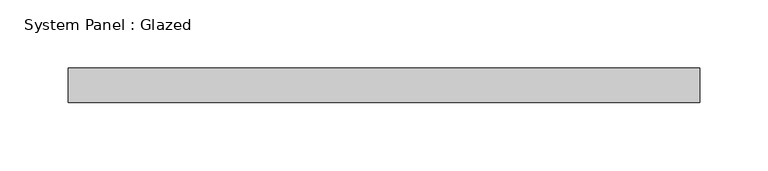
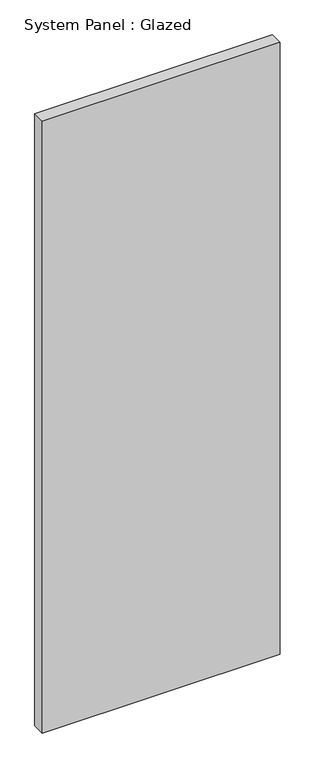
"""IFC4 building model written with IfcOpenShell, lengths in millimetres: plate geometry, System Panel : Glazed."""

from ifc_helpers import new_model, si_unit, origin, origin_with_axes, place, context, project, spatial, polyline, outline, extrude, source, transform, mapped, element, save


def system_panel_glazed_28e9ce38(model_context):
    return source(origin(), model_context, "Body", "SweptSolid", [
        extrude(outline(polyline([(231.775, 19.05), (-231.775, 19.05), (-231.775, 44.45), (231.775, 44.45), (231.775, 19.05)])), origin_with_axes(), (0.0, 0.0, 1.0), 1261.8321364),
    ])


if __name__ == "__main__":
    model = new_model("IFC4")
    model_context = context("Model", 3, world=origin())
    ifc_project = project(units=[si_unit("LENGTHUNIT", "METRE", prefix="MILLI")], contexts=[model_context])
    site = spatial("IfcSite", under=ifc_project)
    building = spatial("IfcBuilding", under=site)
    placement = place(None, origin())
    system_panel_glazed_shape = system_panel_glazed_28e9ce38(model_context)
    element("IfcPlate", 1, ObjectType="System Panel : Glazed", at=placement, inside=building, context=model_context, shape_type="MappedRepresentation", body=[
        mapped(system_panel_glazed_shape, transform((0.0, 0.0, 0.0), x_axis=(1.0, 0.0, 0.0), y_axis=(0.0, 1.0, 0.0), z_axis=(0.0, 0.0, 1.0))),
    ])
    save(model, "model.ifc")

# Revit data of these elements
# Type "System Panel : Glazed"
#   Construction Type Id = "GSP4R"
#   Analytic Construction = "1/8 in Pilkington single glazing"
#   Visual Light Transmittance = 0.9
#   Solar Heat Gain Coefficient = 0.86
#   Heat Transfer Coefficient (U) = 1.18115 BTU/(h·ft²·°F)
#   Define Thermal Properties by = 1
# Element 1 (IfcPlate, "System Panel : Glazed")
#   Materials on its faces: "Glass"
# Materials
#   "Glass": class "Glass", colour RGB 0 128 192, transparency 0.75, Description = "Soda Lime Glass", Cost = 0
